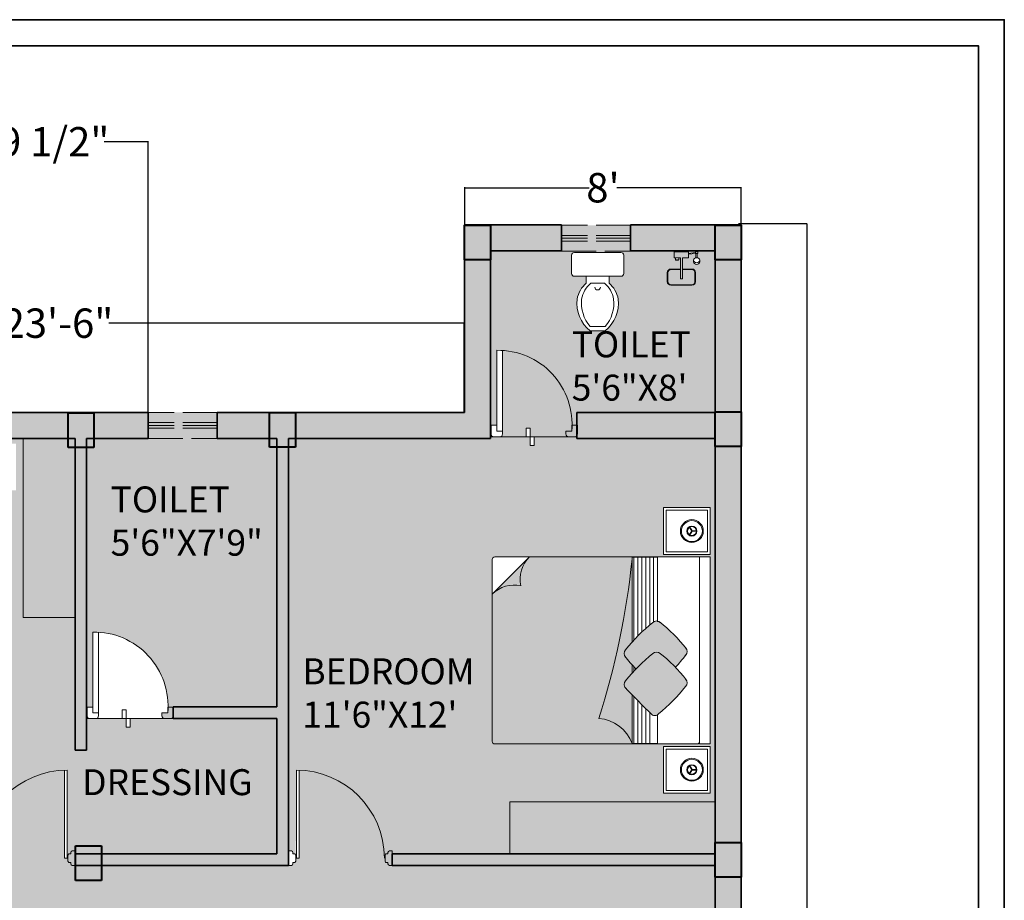
# Model space of a CAD drawing. Units: inches. Extents: x 1077 to 2505, y 1892 to 2728.
# Tile 26 of 26: x 2164 to 2505, y 2423 to 2728. Entities that reach past the tile are written whole.
import ezdxf

# ---------------------------------------------------------------- set-up
doc = ezdxf.new("R2010")
doc.units = ezdxf.units.IN
doc.linetypes.add('ACAD_ISO02W100', pattern=[15, 12, -3])
doc.layers.get('Defpoints').update_dxf_attribs({"color": 220, "linetype": 'ACAD_ISO02W100'})
for name, color, linetype, lineweight in [('00 FURNITURE', 15, 'Continuous', 15), ('A-ANNO-DIMS', 2, 'Continuous', 18), ('A-ANNO-TTLB', 7, 'Continuous', 35), ('A-AREA-IDEN', 7, 'Continuous', 18), ('A-COLS', 7, 'Continuous', 40), ('A-DOOR', 4, 'Continuous', 18), ('A-FLOR-CASE', 8, 'Continuous', 18), ('A-FLOR-FIXT', 8, 'Continuous', 13), ('A-GLAZ-VENT', 6, 'ACAD_ISO02W100', 13), ('A-WALL-PATT', 7, 'Continuous', 9), ('A_FUR 1', 5, 'Continuous', 5), ('WALL', 7, 'Continuous', 35)]:
    doc.layers.add(name, color=color, linetype=linetype, lineweight=lineweight)
for name, color, linetype, lineweight, true_color in [('A-FLOR-CASE-PATT', 32, 'Continuous', 9, 0xcd6928), ('A-FLOR-PATT', 254, 'Continuous', 9, 0xd7ebd2), ('A-FURN-PATT', 177, 'Continuous', 9, 0x293189)]:
    doc.layers.add(name, color=color, linetype=linetype, lineweight=lineweight, true_color=true_color)
doc.styles.get("Standard").update_dxf_attribs({"font": 'arial.ttf'})
doc.dimstyles.get("Standard").update_dxf_attribs({"dimtxt": 10.18, "dimasz": 0.18, "dimexe": 0.18, "dimexo": 0.0625, "dimgap": 0.09, "dimtad": 0, "dimtih": 1, "dimtoh": 1, "dimdec": 0, "dimzin": 0, "dimdsep": 46, "dimlunit": 3, "dimtxsty": 'Standard', "dimcen": 0.09, "dimadec": 0, "dimazin": 0, "dimtfac": 1, "dimtdec": 0, "dimtofl": 0, "dimtmove": 0, "dimatfit": 3, "dimfxl": 1, "dimtolj": 1, "dimtzin": 0, "dimarcsym": 0})

# ---------------------------------------------------------------- blocks, each defined once
blk = doc.blocks.new('*D20')
at = {"layer": 'A-ANNO-DIMS', "color": 0, "lineweight": -2, "transparency": 16777216}
for p, q in [((2317.98, 2657.32), (2317.98, 2670.23)), ((2318.16, 2670.05), (2361.12, 2670.05)), ((2413.64, 2670.05), (2370.68, 2670.05)), ((2413.82, 2657.32), (2413.82, 2670.23))]:
    blk.add_line(p, q, dxfattribs=at)
at = {"layer": 'A-ANNO-DIMS', "color": 0, "transparency": 16777216}
for points in [[(2318.16, 2670.08), (2318.16, 2670.02), (2317.98, 2670.05)], [(2413.64, 2670.08), (2413.64, 2670.02), (2413.82, 2670.05)]]:
    blk.add_solid(points, dxfattribs=at)
at = {"layer": 'Defpoints', "color": 0, "transparency": 16777216}
for p in [(2413.82, 2670.05), (2317.98, 2657.26), (2413.82, 2657.26)]:
    blk.add_point(p, dxfattribs=at)
at = {"layer": 'A-ANNO-DIMS', "color": 0, "transparency": 16777216, "insert": (2365.9, 2670.05), "char_height": 10.18, "attachment_point": 5}
blk.add_mtext("\\A1;8'", dxfattribs=at)
blk = doc.blocks.new('DDD')
at = {"layer": '00 FURNITURE'}
for p, q in [((-12579.77, -15859.53), (-12579.77, -15829.05)), ((-12578.77, -15859.53), (-12578.77, -15829.03)), ((-12612.02, -15857.03), (-12612.02, -15862.03)), ((-12611.02, -15857.03), (-12612.02, -15857.03)), ((-12610.52, -15858.03), (-12610.52, -15857.53)), ((-12577.52, -15858.03), (-12577.52, -15857.53)), ((-12577.02, -15857.03), (-12576.02, -15857.03)), ((-12576.02, -15857.03), (-12576.02, -15862.03)), ((-12610.52, -15861.53), (-12610.52, -15861.03)), ((-12578.77, -15859.53), (-12579.77, -15859.53)), ((-12577.52, -15861.53), (-12577.52, -15861.03)), ((-12612.02, -15862.03), (-12611.02, -15862.03)), ((-12576.02, -15862.03), (-12577.02, -15862.03))]:
    blk.add_line(p, q, dxfattribs=at)
for points in [[(-12610.52, -15861.03), (-12610.02, -15861.03, 0.414214), (-12609.52, -15860.53), (-12609.52, -15858.53, 0.414214), (-12610.02, -15858.03), (-12610.52, -15858.03)], [(-12577.52, -15861.03), (-12578.02, -15861.03, -0.414214), (-12578.52, -15860.53), (-12578.52, -15858.53, -0.414214), (-12578.02, -15858.03), (-12577.52, -15858.03)]]:
    blk.add_lwpolyline(points, format="xyb", dxfattribs=at)
for centre, radius, start, end in [((-12578.77, -15859.53), 30.5, 90, 180), ((-12611.02, -15857.53), 0.5, 0, 90), ((-12577.02, -15857.53), 0.5, 90, 180), ((-12611.02, -15861.53), 0.5, 270, 0), ((-12577.02, -15861.53), 0.5, 180, 270)]:
    blk.add_arc(centre, radius, start, end, dxfattribs=at)
blk = doc.blocks.new('ESTSET')
at = {"layer": 'A_FUR 1'}
for p, q in [((-10.44, 4.1), (-10.44, 32.1)), ((-8.44, 4.1), (-8.44, 32.1)), ((-36.44, 6.1), (-36.44, 3.1)), ((-34.44, 6.1), (-36.44, 6.1)), ((-34.44, 4.1), (-34.44, 6.1)), ((-34.44, 4.1), (-34.44, 6.1)), ((-32.44, 4.1), (-34.44, 4.1)), ((-32.44, 4.1), (-34.44, 4.1)), ((-32.44, 3.1), (-32.44, 4.1)), ((-10.44, 3.1), (-10.44, 4.1)), ((-10.44, 4.1), (-8.44, 4.1)), ((-10.44, 4.1), (-8.44, 4.1)), ((-8.44, 4.1), (-8.44, 6.1)), ((-8.44, 6.1), (-6.44, 6.1)), ((-8.44, 4.1), (-8.44, 6.1)), ((-6.44, 6.1), (-6.44, 3.1)), ((-6.44, 2.1), (-36.44, 2.1)), ((-35.44, 2.1), (-33.44, 2.1)), ((-7.44, 2.1), (-9.44, 2.1))]:
    blk.add_line(p, q, dxfattribs=at)
for points in [[(-21.44, 2.1), (-18.67, 2.1), (-18.67, 5.1), (-20.06, 5.1)], [(-20.06, 5.1), (-20.06, -0.91)], [(-21.44, 2.1), (-21.44, -0.91), (-20.06, -0.91)]]:
    blk.add_lwpolyline(points, dxfattribs=at)
for centre, radius, start, end in [((-8.91, 6.46), 25.64, 88.9606, 185.2816), ((-35.44, 3.1), 1, 180, 270), ((-33.44, 3.1), 1, 270, 0), ((-9.44, 3.1), 1, 180, 270), ((-7.44, 3.1), 1, 270, 0)]:
    blk.add_arc(centre, radius, start, end, dxfattribs=at)
blk = doc.blocks.new('A$C2AC94788')
for p, q in [((0, 0.505), (0, 0.665)), ((0.025, 0.69), (0.435, 0.69)), ((0.46, 0.665), (0.46, 0.505)), ((0.435, 0.48), (0.025, 0.48)), ((0.13, 0.48), (0.13, 0.42)), ((0.33, 0.42), (0.33, 0.48)), ((0.17, 0.42), (0.29, 0.42)), ((0.1641, 0.0392), (0.2959, 0.0392)), ((0.2291, 0.0392), (0.23, 0.0392)), ((0.2309, 0.0392), (0.23, 0.0392)), ((0.165, 0), (0.295, 0))]:
    blk.add_line(p, q)
for centre, radius, start, end in [((0.025, 0.665), 0.025, 90, 180), ((0.435, 0.665), 0.025, 0, 90), ((0.025, 0.505), 0.025, 180, 270), ((0.435, 0.505), 0.025, 270, 0), ((0.2874, 0.2356), 0.2425, 130.48854, 169.44501), ((0.3274, 0.2356), 0.2425, 130.48854, 169.44501), ((0.23, 0.385), 0.025, 180, 0), ((0.1326, 0.2356), 0.2425, 10.55499, 49.51146), ((0.1726, 0.2356), 0.2425, 10.55499, 49.51146), ((0.3601, 0.2448), 0.313, 173.53688, 231.44828), ((0.4001, 0.2448), 0.313, 173.53688, 221.06038), ((0.0999, 0.2448), 0.313, 308.55172, 6.46312), ((0.0599, 0.2448), 0.313, 318.93962, 6.46312)]:
    blk.add_arc(centre, radius, start, end)
blk = doc.blocks.new('A$C7A0926BE')
for p, q in [((-6.55, 0), (-5.57, 0)), ((-6.55, -0.65), (-6.55, 0)), ((-5.57, 0), (-5.57, -0.65)), ((-2.89, 0), (-2.89, -2.29)), ((2.89, 0), (-2.89, 0)), ((2.89, -2.29), (2.89, 0)), ((-7.32, -3.29), (-7.32, -3.94)), ((-5.57, -0.65), (-6.55, -0.65)), ((-6.34, -0.65), (-5.74, -0.65)), ((-6.34, -2.33), (-6.34, -0.65)), ((-5.74, -2.33), (-6.34, -2.33)), ((-5.74, -0.65), (-5.74, -2.33)), ((-5.57, -0.28), (-2.89, -0.56)), ((-5.57, -0.65), (-2.89, -0.94)), ((-4.84, -3.94), (-4.85, -3.29)), ((-2.89, -2.29), (-0.45, -2.29)), ((0.39, -2.29), (2.89, -2.29)), ((1.04, -2.29), (1.04, -3.12)), ((2.37, -2.29), (1.04, -2.29)), ((1.04, -3.12), (2.37, -3.12)), ((1.13, -3.12), (1.13, -3.23)), ((2.3, -3.12), (1.13, -3.12)), ((1.13, -3.23), (2.3, -3.23)), ((2.3, -3.23), (2.3, -3.12)), ((2.37, -3.12), (2.37, -2.29))]:
    blk.add_line(p, q)
at = {"ltscale": 100}
for p, q in [((-0.45, -10.48), (-0.45, -2.29)), ((0.39, -10.48), (0.39, -2.29)), ((0.18, -10.69), (-0.24, -10.69))]:
    blk.add_line(p, q, dxfattribs=at)
for points in [[(-0.45, -6.79), (-4.23, -6.79, 0.414214), (-5.63, -8.19), (-5.63, -11.8, 0.414214), (-4.23, -13.2), (4.17, -13.2, 0.414214), (5.57, -11.8), (5.57, -8.19, 0.414214), (4.17, -6.79), (0.39, -6.79)], [(-0.45, -7), (-4.23, -7, 0.414214), (-5.42, -8.19), (-5.42, -11.8, 0.414214), (-4.23, -12.99), (4.17, -12.99, 0.414214), (5.36, -11.8), (5.36, -8.19, 0.414214), (4.17, -7), (0.39, -7)]]:
    blk.add_lwpolyline(points, format="xyb", dxfattribs=at)
for centre, start, end in [((-0.24, -10.48), 180, 270), ((0.18, -10.48), 270, 0)]:
    blk.add_arc(centre, 0.21, start, end, dxfattribs=at)
at = {"extrusion": (0, 0, -1)}
blk.add_ellipse((-6.08, -3.29), major_axis=(-1.24, 0), ratio=0.790849, dxfattribs=at)
blk.add_ellipse((-6.08, -3.94), major_axis=(-1.24, 0), ratio=0.790849, start_param=3.141593, end_param=6.283185, dxfattribs=at)
blk = doc.blocks.new('RGWTG')
at = {"layer": '00 FURNITURE'}
for p, q in [((578.23, 3473.51), (577.36, 3475.01)), ((578.23, 3473.58), (577.36, 3472.08)), ((578.36, 3473.58), (577.49, 3475.09)), ((578.36, 3473.51), (577.49, 3472)), ((578.29, 3473.62), (580.03, 3473.62)), ((578.29, 3473.47), (580.03, 3473.47)), ((521.93, 3464.58), (509.03, 3451.68)), ((509.03, 3422.63), (509.03, 3463.68)), ((509.93, 3464.58), (566.4, 3464.58)), ((557.53, 3463.84), (557.53, 3464.49)), ((557.53, 3464.49), (566.4, 3464.49)), ((558.2, 3464.49), (558.2, 3435.82)), ((559.57, 3464.49), (559.57, 3437.25)), ((560.94, 3464.49), (560.94, 3438.58)), ((562.3, 3464.49), (562.3, 3439.83)), ((563.67, 3464.49), (563.67, 3440.99)), ((565.04, 3464.49), (565.04, 3442.08)), ((566.4, 3464.58), (580.98, 3464.58)), ((566.4, 3464.49), (566.4, 3442.08)), ((566.4, 3464.49), (566.4, 3463.84)), ((580.98, 3464.58), (580.98, 3416.72)), ((558.2, 3426.48), (558.2, 3425.04)), ((509.03, 3400.68), (509.03, 3422.63)), ((558.2, 3416.13), (558.2, 3399.95)), ((559.57, 3414.75), (559.57, 3399.95)), ((580.98, 3416.72), (580.98, 3400.68)), ((560.94, 3413.39), (560.94, 3399.95)), ((562.3, 3412.04), (562.3, 3399.95)), ((563.67, 3410.72), (563.67, 3399.95)), ((580.08, 3399.78), (509.93, 3399.78)), ((557.53, 3399.95), (557.53, 3400.6)), ((566.4, 3399.95), (557.53, 3399.95)), ((566.4, 3400.6), (566.4, 3399.95)), ((578.23, 3390.78), (577.36, 3392.29)), ((578.23, 3390.86), (577.36, 3389.36)), ((578.36, 3390.86), (577.49, 3392.36)), ((578.29, 3390.9), (580.03, 3390.9)), ((578.36, 3390.78), (577.49, 3389.28)), ((578.29, 3390.74), (580.03, 3390.74))]:
    blk.add_line(p, q, dxfattribs=at)
for points in [[(568.43, 3465.48), (584.63, 3465.48), (584.63, 3481.68), (568.43, 3481.68)], [(569.33, 3466.38), (583.73, 3466.38), (583.73, 3480.78), (569.33, 3480.78)], [(580.98, 3399.78), (584.63, 3399.78), (584.63, 3464.58), (580.98, 3464.58)], [(568.43, 3398.88), (584.63, 3398.88), (584.63, 3382.68), (568.43, 3382.68)], [(569.33, 3397.98), (583.73, 3397.98), (583.73, 3383.58), (569.33, 3383.58)]]:
    blk.add_lwpolyline(points, close=True, dxfattribs=at)
for points in [[(566.52, 3464.49), (557.53, 3464.49), (557.53, 3435.08)], [(557.53, 3427.21), (557.53, 3424.3)], [(557.53, 3416.82), (557.53, 3399.95), (566.4, 3399.95), (566.4, 3409.94)]]:
    blk.add_lwpolyline(points, dxfattribs=at)
for centre, radius in [((578.29, 3473.54), 3.97), ((578.29, 3473.54), 3.63), ((578.29, 3473.54), 1.74), ((578.29, 3473.54), 1.56), ((578.29, 3390.82), 3.97), ((578.29, 3390.82), 3.63), ((578.29, 3390.82), 1.74), ((578.29, 3390.82), 1.56)]:
    blk.add_circle(centre, radius, dxfattribs=at)
for centre, radius, start, end in [((509.93, 3463.68), 0.9, 90, 180), ((529.65, 3456.88), 10.9, 135.0361, 191.9278), ((290.56, 3490.52), 268.3, 342.2214, 354.2925), ((516.73, 3443.97), 10.9, 78.0722, 134.9639), ((566.05, 3440.57), 1.82, 45, 135), ((533.58, 3399.31), 54.32, 37.931, 52.069), ((598.15, 3399.01), 54.32, 127.931, 142.069), ((556.59, 3431.11), 1.82, 135, 225), ((574.84, 3431.77), 1.82, 315, 45), ((597.87, 3463.6), 54.32, 217.931, 224.141), ((598.15, 3388.23), 54.32, 127.931, 142.069), ((566.05, 3429.78), 1.82, 45, 135), ((533.58, 3388.53), 54.32, 37.931, 52.069), ((533.28, 3463.88), 54.32, 316.32, 322.069), ((556.59, 3420.33), 1.82, 135, 225), ((574.84, 3420.99), 1.82, 315, 45), ((765.33, 3619.75), 290.45, 223.6069, 226.2326), ((533.28, 3453.1), 54.32, 307.931, 322.069), ((545.02, 3395.29), 13.35, 20.4224, 85.5825), ((565.44, 3411.05), 1.47, 225.9674, 326.8337), ((509.93, 3400.68), 0.9, 180, 270), ((580.08, 3400.68), 0.9, 270, 0)]:
    blk.add_arc(centre, radius, start, end, dxfattribs=at)
blk = doc.blocks.new('C1')
h = blk.add_hatch(color=256)
h.dxf.hatch_style = 1
h.paths.add_polyline_path([(1668.56, 2445.41), (1677.56, 2445.41), (1677.56, 2457.41), (1668.56, 2457.41)])
for p, q in [((1668.56, 2457.41), (1677.56, 2457.41)), ((1668.56, 2445.41), (1668.56, 2457.41)), ((1677.56, 2457.41), (1677.56, 2445.41)), ((1677.56, 2445.41), (1668.56, 2445.41))]:
    blk.add_line(p, q)
blk = doc.blocks.new('*D18')
at = {"layer": 'A-ANNO-DIMS', "color": 0, "lineweight": -2, "transparency": 16777216}
for p, q in [((2035.96, 2592.42), (2035.96, 2623.29)), ((2036.14, 2623.11), (2159.23, 2623.11)), ((2317.64, 2623.11), (2194.55, 2623.11)), ((2317.82, 2592.42), (2317.82, 2623.29))]:
    blk.add_line(p, q, dxfattribs=at)
at = {"layer": 'A-ANNO-DIMS', "color": 0, "transparency": 16777216}
for points in [[(2036.14, 2623.14), (2036.14, 2623.08), (2035.96, 2623.11)], [(2317.64, 2623.14), (2317.64, 2623.08), (2317.82, 2623.11)]]:
    blk.add_solid(points, dxfattribs=at)
at = {"layer": 'Defpoints', "color": 0, "transparency": 16777216}
for p in [(2317.82, 2623.11), (2035.96, 2592.36), (2317.82, 2592.36)]:
    blk.add_point(p, dxfattribs=at)
at = {"layer": 'A-ANNO-DIMS', "color": 0, "transparency": 16777216, "insert": (2176.89, 2623.11), "char_height": 10.18, "attachment_point": 5}
blk.add_mtext('\\A1;23\'-6"', dxfattribs=at)
blk = doc.blocks.new('*D19')
at = {"layer": 'A-ANNO-DIMS', "color": 0, "lineweight": -2, "transparency": 16777216}
for p, q in [((2412.91, 2657.64), (2436.75, 2657.64)), ((2436.57, 2657.46), (2436.57, 2381.28)), ((2436.57, 2094.52), (2436.57, 2370.7)), ((2412.91, 2094.34), (2436.75, 2094.34))]:
    blk.add_line(p, q, dxfattribs=at)
at = {"layer": 'A-ANNO-DIMS', "color": 0, "transparency": 16777216}
for points in [[(2436.54, 2657.46), (2436.6, 2657.46), (2436.57, 2657.64)], [(2436.54, 2094.52), (2436.6, 2094.52), (2436.57, 2094.34)]]:
    blk.add_solid(points, dxfattribs=at)
at = {"layer": 'Defpoints', "color": 0, "transparency": 16777216}
for p in [(2412.85, 2657.64), (2412.85, 2094.34), (2436.57, 2094.34)]:
    blk.add_point(p, dxfattribs=at)
at = {"layer": 'A-ANNO-DIMS', "color": 0, "transparency": 16777216, "insert": (2436.57, 2375.99), "char_height": 10.18, "attachment_point": 5}
blk.add_mtext('\\A1;46\'-11"', dxfattribs=at)
blk = doc.blocks.new('VENT-24')
for p, q in [((3.5, 24), (3.5, 0)), ((4.5, 24), (4.5, 0)), ((5.5, 24), (5.5, 0))]:
    blk.add_line(p, q)
blk.add_lwpolyline([(0, 0), (9, 0), (9, 24), (0, 24)], close=True)
blk = doc.blocks.new('SHEET-FRAME-RESIDENTIAL')
for points in [[(0, 830.04), (543.52, 830.04), (543.52, 0), (0, 0)], [(9, 821.04), (534.52, 821.04), (534.52, 9), (9, 9)]]:
    blk.add_lwpolyline(points, close=True)
blk = doc.blocks.new('*D48')
at = {"layer": 'A-ANNO-DIMS', "color": 0, "lineweight": -2, "transparency": 16777216}
for p, q in [((2256.78, 2416.24), (2259.43, 2416.24)), ((2259.25, 2416.06), (2259.25, 2413.13)), ((2259.25, 2399.49), (2259.25, 2402.42)), ((2256.78, 2399.31), (2259.43, 2399.31))]:
    blk.add_line(p, q, dxfattribs=at)
at = {"layer": 'A-ANNO-DIMS', "color": 0, "transparency": 16777216}
for points in [[(2259.22, 2416.06), (2259.28, 2416.06), (2259.25, 2416.24)], [(2259.22, 2399.49), (2259.28, 2399.49), (2259.25, 2399.31)]]:
    blk.add_solid(points, dxfattribs=at)
at = {"layer": 'Defpoints', "color": 0, "transparency": 16777216}
for p in [(2256.72, 2416.24), (2259.25, 2416.24), (2256.72, 2399.31)]:
    blk.add_point(p, dxfattribs=at)
at = {"layer": 'A-ANNO-DIMS', "color": 0, "transparency": 16777216, "insert": (2259.25, 2407.77), "char_height": 10.18, "attachment_point": 5}
blk.add_mtext('\\A1;DINING CHAIR 1\'-5" TYP.', dxfattribs=at)
blk = doc.blocks.new('*D74')
at = {"layer": 'A-ANNO-DIMS', "color": 0, "lineweight": -2, "transparency": 16777216}
for p, q in [((2126.63, 2592.2), (2126.63, 2686.17)), ((2126.81, 2685.99), (2141.88, 2685.99)), ((2207.97, 2685.99), (2192.9, 2685.99)), ((2208.15, 2592.2), (2208.15, 2686.17))]:
    blk.add_line(p, q, dxfattribs=at)
at = {"layer": 'A-ANNO-DIMS', "color": 0, "transparency": 16777216}
for points in [[(2126.81, 2686.02), (2126.81, 2685.96), (2126.63, 2685.99)], [(2207.97, 2686.02), (2207.97, 2685.96), (2208.15, 2685.99)]]:
    blk.add_solid(points, dxfattribs=at)
at = {"layer": 'Defpoints', "color": 0, "transparency": 16777216}
for p in [(2208.15, 2685.99), (2126.63, 2592.14), (2208.15, 2592.14)]:
    blk.add_point(p, dxfattribs=at)
at = {"layer": 'A-ANNO-DIMS', "color": 0, "transparency": 16777216, "insert": (2167.39, 2685.99), "char_height": 10.18, "attachment_point": 5}
blk.add_mtext('\\A1;6\'-9 1/2"', dxfattribs=at)

msp = doc.modelspace()

# ---------------------------------------------------------------- hatches: boundary and pattern name
at = {"layer": 'A-FLOR-CASE-PATT', "transparency": 33554610}
h = msp.add_hatch(color=256, dxfattribs=at)
h.dxf.hatch_style = 1
h.paths.add_polyline_path([(2182.85, 2583.13), (2164.84, 2583.13), (2164.84, 2521.11), (2182.85, 2521.11)])
h.paths.add_polyline_path([(2333.66, 2457.16), (2333.66, 2439.14), (2404.85, 2439.14), (2404.85, 2443.09), (2404.85, 2457.16)])
at = {"layer": 'A-FLOR-PATT', "transparency": 33554559}
h = msp.add_hatch(color=256, dxfattribs=at)
h.dxf.hatch_style = 1
h.paths.add_polyline_path([(2252.85, 2583.14), (2232.15, 2583.14), (2208.15, 2583.17), (2208.15, 2583.14), (2186.85, 2583.14), (2186.85, 2486.14), (2186.85, 2475.14), (2182.85, 2475.14), (2182.85, 2521.11), (2164.84, 2521.11), (2164.84, 2583.14), (2126.63, 2583.14), (2078.63, 2583.13), (2078.63, 2583.14), (2044.85, 2583.14), (2044.85, 2439.14), (2146.85, 2439.14), (2146.85, 2435.14), (2120.85, 2435.14), (2044.85, 2435.14), (2044.85, 2401), (2044.85, 2401), (2044.85, 2377), (2044.85, 2377), (2044.85, 2313.14), (2116.85, 2313.14), (2116.85, 2405.14), (2120.85, 2405.14), (2120.85, 2313.14), (2146.85, 2313.14), (2146.85, 2312.21), (2182.85, 2312.21), (2182.85, 2313.14), (2186.85, 2313.14), (2186.85, 2312.21), (2222.85, 2312.21), (2222.85, 2313.14), (2289.85, 2313.14), (2289.85, 2094.14), (2404.85, 2094.14), (2404.85, 2146.06), (2368.85, 2146.06), (2368.85, 2273.14), (2332.85, 2273.14), (2332.85, 2309.14), (2325.85, 2309.14), (2325.85, 2313.14), (2404.85, 2313.14), (2404.85, 2354.2), (2404.85, 2402.2), (2404.85, 2435.14), (2292.85, 2435.14), (2292.85, 2439.14), (2333.66, 2439.14), (2333.66, 2457.16), (2404.85, 2457.16), (2404.85, 2583.14), (2356.85, 2583.14), (2356.85, 2592.14), (2404.85, 2592.14), (2404.85, 2648.14), (2375.5, 2648.14), (2375.5, 2648.03), (2351.47, 2648.03), (2351.47, 2648.14), (2326.85, 2648.14), (2326.85, 2583.14), (2256.85, 2583.14), (2256.85, 2435.14), (2182.85, 2435.14), (2182.85, 2439.14), (2186.85, 2439.14), (2252.85, 2439.14), (2252.85, 2486.14), (2216.85, 2486.14), (2216.85, 2490.14), (2252.85, 2490.14)])
h.paths.add_polyline_path([(2214.97, 2488.05), (2212.97, 2488.05), (2212.97, 2487.05, 0.414214), (2213.97, 2486.05), (2201.97, 2486.05), (2201.97, 2483.04), (2200.58, 2483.04), (2200.58, 2486.05), (2187.97, 2486.05, -0.414214), (2186.97, 2487.05), (2186.97, 2490.05), (2188.97, 2490.05), (2188.97, 2516.05, -0.446908)], flags=16)
h.paths.add_polyline_path([(2162.4, 2565.16), (2146.2, 2565.16), (2146.2, 2581.36), (2162.4, 2581.36)], flags=16)
h.paths.add_polyline_path([(2161.5, 2566.06), (2147.1, 2566.06), (2147.1, 2580.46), (2161.5, 2580.46)], flags=0)
h.paths.add_polyline_path([(2145.3, 2506.66, -0.414214), (2144.4, 2505.76), (2122.45, 2505.76), (2081.4, 2505.76, -0.414214), (2080.5, 2506.66), (2080.5, 2563.14), (2080.5, 2577.72), (2080.5, 2581.36), (2145.3, 2581.36), (2145.3, 2577.72), (2144.4, 2577.72, -0.414214), (2145.3, 2576.82)], flags=16)
h.paths.add_polyline_path([(2150.3, 2575.03, -1), (2158.24, 2575.03, -1)], flags=0)
h.paths.add_polyline_path([(2150.64, 2575.03, -1), (2157.89, 2575.03, -1)], flags=0)
h.paths.add_polyline_path([(2180.11, 2468.19), (2180.11, 2437.69), (2180.36, 2436.69), (2180.36, 2437.69), (2179.11, 2437.69), (2179.11, 2468.17, 0.404641), (2149.61, 2437.69), (2149.36, 2436.69, -0.414214), (2148.86, 2436.19), (2148.36, 2436.19), (2148.36, 2435.69, -0.414214), (2147.86, 2435.19), (2146.86, 2435.19), (2146.86, 2440.19), (2147.86, 2440.19, -0.414214), (2148.36, 2439.69), (2148.36, 2439.19), (2148.86, 2439.19, -0.414214), (2149.36, 2438.69), (2149.61, 2437.69, -0.414214)], flags=16)
h.paths.add_polyline_path([(2145.14, 2554.26, 0.292232), (2136.49, 2542.78, 0.052719), (2081.25, 2554.26), (2080.6, 2554.26), (2080.6, 2563.14), (2081.25, 2563.14), (2102.73, 2563.14, -0.117785), (2103.09, 2563.91, -0.059418), (2112.19, 2573, -0.379859), (2114.6, 2572.86, -0.02509), (2118.73, 2569.3, -0.025935), (2122.97, 2573, -0.379859), (2125.38, 2572.86, -0.061767), (2134.84, 2563.41, -0.069393), (2135.14, 2563.14), (2145.14, 2563.14)], flags=0)
h.paths.add_polyline_path([(2120.79, 2554.26), (2117.88, 2554.26, -0.015371), (2115.33, 2552.11, -0.429576), (2112.69, 2552.04, -0.016036), (2110.01, 2554.26), (2080.6, 2554.26), (2080.6, 2560.4), (2104.1, 2560.4, 0.055344), (2112.69, 2552.04, 0.331768), (2114.84, 2551.72, 0.027343), (2119.32, 2555.62, 0.00919)], flags=0)
h.paths.add_polyline_path([(2152.88, 2574.32), (2154.19, 2575.07), (2154.19, 2576.58, 0.399698), (2152.71, 2575.03, 0.119004)], flags=0)
h.paths.add_polyline_path([(2152.53, 2575.03, -1), (2156, 2575.03, -1)], flags=0)
h.paths.add_polyline_path([(2154.27, 2574.94), (2154.34, 2574.98), (2154.34, 2575.07), (2154.3, 2575.09), (2154.23, 2574.96)], flags=0)
h.paths.add_polyline_path([(2259.6, 2468.17, -0.414214), (2290.1, 2437.67), (2290.35, 2438.67), (2290.1, 2437.67, 0.404641), (2260.6, 2468.15), (2260.6, 2437.67), (2259.35, 2437.67), (2259.35, 2436.67, -0.414214), (2258.85, 2436.17), (2258.35, 2436.17), (2258.35, 2435.67, -0.414214), (2257.85, 2435.17), (2256.85, 2435.17), (2256.85, 2440.17), (2257.85, 2440.17, -0.414214), (2258.35, 2439.67), (2258.35, 2439.17), (2258.85, 2439.17, -0.414214), (2259.35, 2438.67)], flags=16)
h.paths.add_polyline_path([(2327.48, 2541.19, -0.414214), (2328.38, 2542.09), (2384.85, 2542.09), (2399.43, 2542.09), (2403.08, 2542.09), (2403.08, 2477.29), (2399.43, 2477.29), (2399.43, 2478.19, -0.414214), (2398.53, 2477.29), (2328.38, 2477.29, -0.414214), (2327.48, 2478.19), (2327.48, 2500.14)], flags=16)
h.paths.add_polyline_path([(2340.38, 2542.09, 0.253465), (2337.43, 2532.13, 0.2538), (2327.47, 2529.17)], flags=16)
h.paths.add_polyline_path([(2080.5, 2518.67, 0.253465), (2090.46, 2515.72, 0.2538), (2093.42, 2505.75)], flags=16)
h.paths.add_polyline_path([(2327.09, 2584.7), (2327.09, 2587.7), (2329.09, 2587.7), (2329.09, 2613.7, -0.01951), (2331.09, 2613.66), (2331.09, 2585.7), (2331.09, 2584.7, -0.414214), (2330.09, 2583.7), (2328.09, 2583.7, -0.414214)], flags=16)
h.paths.add_polyline_path([(2239.78, 2404.11), (2252.36, 2404.11), (2252.36, 2405.72), (2239.78, 2405.72)], flags=16)
h.paths.add_polyline_path([(2237.26, 2403.16), (2237.26, 2395.8), (2237.82, 2395.8), (2237.82, 2402.03, -0.41429), (2238.38, 2402.59), (2253.79, 2402.59, -0.414213), (2254.35, 2402.03), (2254.35, 2395.8), (2254.91, 2395.8), (2254.91, 2403.16)], flags=16)
h.paths.add_polyline_path([(2120.69, 2434.12), (2120.69, 2432.12, -0.414214), (2119.69, 2431.12), (2118.69, 2431.12), (2090.73, 2431.12, 0.400854), (2116.69, 2407.02), (2116.69, 2407.12), (2118.69, 2407.12, -0.446908), (2090.69, 2433.12), (2116.69, 2433.12), (2116.69, 2435.12), (2119.69, 2435.12, -0.414214)], flags=16)
h.paths.add_polyline_path([(2262.11, 2404.11), (2274.69, 2404.11), (2274.69, 2405.72), (2262.11, 2405.72)], flags=16)
h.paths.add_polyline_path([(2259.59, 2403.16), (2262.11, 2404.11), (2274.69, 2404.11), (2277.24, 2403.16)], flags=16)
h.paths.add_polyline_path([(2289.58, 2389.14), (2289.58, 2376.57), (2291.19, 2376.57), (2291.19, 2389.14)], flags=16)
h.paths.add_polyline_path([(2288.62, 2391.67), (2281.15, 2391.67), (2281.15, 2391.11), (2287.5, 2391.11, -0.41429), (2288.06, 2390.54), (2288.06, 2375.14, -0.414237), (2287.5, 2374.58), (2281.15, 2374.58), (2281.15, 2374.01), (2288.62, 2374.01)], flags=16)
h.paths.add_polyline_path([(2274.69, 2357.14), (2274.69, 2355.52), (2276.22, 2355.52, 0.414236), (2277.24, 2356.54), (2277.24, 2358.09)], flags=16)
h.paths.add_polyline_path([(2252.36, 2357.14), (2252.36, 2355.52), (2253.89, 2355.52, 0.414235), (2254.91, 2356.54), (2254.91, 2358.09)], flags=16)
h.paths.add_polyline_path([(2224.02, 2376.03), (2222.41, 2376.03), (2222.41, 2374.5, 0.414235), (2223.43, 2373.48), (2224.98, 2373.48)], flags=16)
h.paths.add_polyline_path([(2276.68, 2365.45), (2276.68, 2359.22, -0.41419), (2276.12, 2358.66), (2260.71, 2358.66, -0.414137), (2260.15, 2359.22), (2260.15, 2365.45), (2254.35, 2365.45), (2254.35, 2359.22, -0.414189), (2253.79, 2358.66), (2238.38, 2358.66, -0.414137), (2237.82, 2359.22), (2237.82, 2365.45)], flags=16)
h.paths.add_polyline_path([(2079.6, 2565.16), (2063.4, 2565.16), (2063.4, 2581.36), (2079.6, 2581.36)], flags=16)
h.paths.add_polyline_path([(2078.7, 2566.06), (2064.3, 2566.06), (2064.3, 2580.46), (2078.7, 2580.46)], flags=0)
h.paths.add_polyline_path([(2339.31, 2583.7), (2339.31, 2586.71), (2340.7, 2586.71), (2340.7, 2583.7), (2342.09, 2583.7), (2342.09, 2580.7), (2340.7, 2580.7), (2340.7, 2583.7)], flags=16)
h.paths.add_polyline_path([(2123.69, 2421.51), (2123.69, 2420.12), (2120.69, 2420.12), (2120.69, 2421.51), (2117.68, 2421.51), (2117.68, 2422.89), (2120.69, 2422.89), (2120.69, 2421.51)], flags=16)
h.paths.add_polyline_path([(2067.57, 2575.03, -1), (2075.51, 2575.03, -1)], flags=0)
h.paths.add_polyline_path([(2067.92, 2575.03, -1), (2075.17, 2575.03, -1)], flags=0)
h.paths.add_polyline_path([(2070.16, 2574.32), (2071.47, 2575.07), (2071.47, 2576.58, 0.399698), (2069.99, 2575.03, 0.119004)], flags=0)
h.paths.add_polyline_path([(2069.81, 2575.03, -1), (2073.28, 2575.03, -1)], flags=0)
h.paths.add_polyline_path([(2071.54, 2574.94), (2071.62, 2574.89), (2071.62, 2574.98)], flags=0)
h.paths.add_polyline_path([(2364.5, 2486.1, 0.052719), (2375.98, 2541.34), (2375.98, 2541.99), (2384.85, 2541.99), (2384.85, 2541.34), (2384.85, 2519.86, -0.117785), (2385.62, 2519.51, -0.059418), (2394.72, 2510.41, -0.379859), (2394.58, 2507.99, -0.02509), (2391.01, 2503.87, -0.025935), (2394.72, 2499.62, -0.379859), (2394.58, 2497.21, -0.061767), (2385.12, 2487.75, -0.069393), (2384.85, 2487.45), (2384.85, 2477.45), (2375.98, 2477.45, 0.292232)], flags=0)
h.paths.add_polyline_path([(2373.75, 2509.9, -0.016036), (2375.98, 2512.58), (2375.98, 2541.99), (2382.12, 2541.99), (2382.12, 2518.49, 0.055344), (2373.75, 2509.9, 0.331768), (2373.44, 2507.75, 0.027343), (2377.33, 2503.27, 0.00919), (2375.98, 2501.8), (2375.98, 2504.71, -0.015371), (2373.82, 2507.26, -0.429576)], flags=0)
h.paths.add_polyline_path([(2356.95, 2631.48, -0.171636), (2360.13, 2636.99), (2360.13, 2639.35), (2356, 2639.35, -0.414214), (2355.01, 2640.34), (2355.01, 2646.64, -0.414214), (2356, 2647.62), (2372.14, 2647.62, -0.414214), (2373.13, 2646.64), (2373.13, 2640.34, -0.414214), (2372.14, 2639.35), (2368.01, 2639.35), (2368.01, 2636.99, -0.171636), (2371.2, 2631.48, -0.258205), (2366.63, 2620.45), (2361.51, 2620.45, -0.258205)], flags=16)
h.paths.add_polyline_path([(2358.52, 2631.48, -0.171636), (2361.71, 2636.99), (2366.43, 2636.99, -0.171636), (2369.62, 2631.48, -0.210384), (2366.67, 2622), (2361.47, 2622, -0.210384)], flags=0)
h.paths.add_polyline_path([(2386.88, 2542.99), (2386.88, 2559.19), (2403.08, 2559.19), (2403.08, 2542.99)], flags=16)
h.paths.add_polyline_path([(2387.78, 2543.89), (2387.78, 2558.29), (2402.18, 2558.29), (2402.18, 2543.89)], flags=0)
h.paths.add_polyline_path([(2392.77, 2551.05, -1), (2400.71, 2551.05, -1)], flags=0)
h.paths.add_polyline_path([(2393.11, 2551.05, -1), (2400.37, 2551.05, -1)], flags=0)
h.paths.add_polyline_path([(2386.88, 2476.39), (2403.08, 2476.39), (2403.08, 2460.19), (2386.88, 2460.19)], flags=16)
h.paths.add_polyline_path([(2398.48, 2550.97), (2398.3, 2550.97, -0.544606), (2396.03, 2549.66), (2395.94, 2549.51, 0.547962)], flags=0)
h.paths.add_polyline_path([(2387.78, 2475.49), (2402.18, 2475.49), (2402.18, 2461.09), (2387.78, 2461.09)], flags=0)
h.paths.add_polyline_path([(2396.79, 2551.12), (2396.74, 2551.2), (2396.7, 2551.12)], flags=0)
h.paths.add_polyline_path([(2400.71, 2468.32, -1), (2392.77, 2468.32, -1)], flags=0)
h.paths.add_polyline_path([(2400.37, 2468.32, -1), (2393.11, 2468.32, -1)], flags=0)
h.paths.add_polyline_path([(2398.48, 2468.25), (2398.3, 2468.25, -0.544606), (2396.03, 2466.94), (2395.94, 2466.78, 0.547962)], flags=0)
h.paths.add_polyline_path([(2396.79, 2468.4), (2396.74, 2468.48), (2396.7, 2468.4)], flags=0)
h.paths.add_polyline_path([(2292.64, 2341.23, -0.414214), (2323.14, 2310.73), (2323.39, 2311.73), (2323.14, 2310.73, 0.404641), (2293.64, 2341.21), (2293.64, 2310.73), (2292.39, 2310.73), (2292.39, 2309.73, -0.414214), (2291.89, 2309.23), (2291.39, 2309.23), (2291.39, 2308.73, -0.414214), (2290.89, 2308.23), (2289.89, 2308.23), (2289.89, 2313.23), (2290.89, 2313.23, -0.414214), (2291.39, 2312.73), (2291.39, 2312.23), (2291.89, 2312.23, -0.414214), (2292.39, 2311.73)], flags=16)
h.paths.add_polyline_path([(2389.45, 2641.69), (2392.75, 2641.69), (2392.75, 2641.87), (2389.45, 2641.87)], flags=16)
edge = h.paths.add_edge_path(flags=16)
edge.add_arc((2393.3, 2638.65), 0.183, 270, 360)
edge.add_line((2393.49, 2638.65), (2393.49, 2645.8))
edge.add_line((2393.49, 2645.8), (2395.61, 2645.8))
edge.add_line((2395.61, 2645.8), (2395.61, 2647.8))
edge.add_line((2395.61, 2647.8), (2390.57, 2647.8))
edge.add_line((2390.57, 2647.8), (2390.57, 2645.8))
edge.add_line((2390.57, 2645.8), (2392.19, 2645.8))
edge.add_line((2392.19, 2645.8), (2392.19, 2644.98))
edge.add_line((2392.19, 2644.98), (2391.02, 2644.98))
edge.add_line((2391.02, 2644.98), (2391.02, 2645.8))
edge.add_line((2391.02, 2645.8), (2390.57, 2645.8))
edge.add_line((2390.57, 2645.8), (2390.57, 2647.8))
edge.add_line((2390.57, 2647.8), (2395.61, 2647.8))
edge.add_line((2395.61, 2647.8), (2395.61, 2647.32))
edge.add_line((2395.61, 2647.32), (2397.95, 2647.56))
edge.add_line((2397.95, 2647.56), (2397.95, 2647.8))
edge.add_line((2397.95, 2647.8), (2398.81, 2647.8))
edge.add_line((2398.81, 2647.8), (2398.81, 2647.23))
edge.add_line((2398.81, 2647.23), (2398.63, 2645.77))
edge.add_ellipse((2398.41, 2644.93), major_axis=(-1.08, 0), ratio=0.790849, start_angle=180, end_angle=255.2976, ccw=False)
edge.add_line((2399.49, 2644.93), (2399.49, 2644.36))
edge.add_ellipse((2398.41, 2644.36), major_axis=(-1.08, 0), ratio=0.790849, start_angle=0, end_angle=180, ccw=False)
edge.add_line((2397.32, 2644.36), (2397.33, 2644.85))
edge.add_ellipse((2398.41, 2644.93), major_axis=(-1.08, 0), ratio=0.790849, start_angle=284.7024, end_angle=364.0401, ccw=False)
edge.add_line((2398.1, 2645.73), (2398.1, 2647.23))
edge.add_line((2398.1, 2647.23), (2397.95, 2647.23))
edge.add_line((2397.95, 2647.23), (2395.61, 2646.99))
edge.add_line((2395.61, 2646.99), (2395.61, 2645.8))
edge.add_line((2395.61, 2645.8), (2393.49, 2645.8))
edge.add_line((2393.49, 2645.8), (2393.49, 2638.46))
edge.add_line((2393.49, 2638.46), (2393.3, 2638.46))
h.paths.add_polyline_path([(2353.64, 2256.32, -0.292371), (2356.22, 2253.81, -0.085148), (2358.52, 2214.83, -0.01331), (2357.59, 2104.48, -0.379287), (2354.54, 2101.26, -0.0502), (2298.86, 2101.26, -0.379287), (2295.81, 2104.48, -0.01331), (2294.88, 2214.83, -0.086132), (2297.28, 2254.24, -0.295116), (2299.9, 2256.76, -0.114238)], flags=16)
h.paths.add_polyline_path([(2352.48, 2211.82, -0.355389), (2354.02, 2208.08), (2350.26, 2195.63, -0.398275), (2346.44, 2193.45, 0.113332), (2306.96, 2193.45, -0.398275), (2303.14, 2195.63), (2299.38, 2208.08, -0.355394), (2300.92, 2211.82, -0.265725)], flags=0)
h.paths.add_polyline_path([(2297.68, 2201.7), (2303.26, 2187.65), (2303.26, 2166.61), (2298.16, 2163.24)], flags=0)
h.paths.add_polyline_path([(2355.78, 2201.7), (2355.31, 2163.24), (2350.2, 2166.61), (2350.2, 2187.65)], flags=0)
h.paths.add_polyline_path([(2303.26, 2164.35), (2303.26, 2143.1), (2298.44, 2128.54), (2298.19, 2161.01)], flags=0)
h.paths.add_polyline_path([(2350.2, 2164.35), (2355.28, 2161.01), (2355.03, 2128.54), (2350.2, 2143.1)], flags=0)
h.paths.add_polyline_path([(2347.2, 2136.38), (2351.71, 2113.65, -0.090102), (2301.76, 2113.63), (2306.27, 2136.37, 0.036636)], flags=0)
h.paths.add_polyline_path([(2304.86, 2165.32), (2354.76, 2165.32), (2354.76, 2183.87), (2304.86, 2183.87)], flags=8)
h.paths.add_polyline_path([(2053.76, 2360.82), (2103.97, 2360.82), (2103.97, 2394.41), (2053.76, 2394.41)], flags=24)
h.paths.add_polyline_path([(2153.41, 2366.23), (2211.12, 2366.23), (2211.12, 2399.82), (2153.41, 2399.82)], flags=24)
h.paths.add_polyline_path([(2258.04, 2477.83), (2327.95, 2477.83), (2327.95, 2511.42), (2258.04, 2511.42)], flags=24)
h.paths.add_polyline_path([(2182.1, 2454.46), (2252.27, 2454.46), (2252.27, 2473), (2182.1, 2473)], flags=24)
h.paths.add_polyline_path([(2192.4, 2537.41), (2246.99, 2537.41), (2246.99, 2571), (2192.4, 2571)], flags=24)
h.paths.add_polyline_path([(2083.07, 2465.98), (2152.99, 2465.98), (2152.99, 2499.56), (2083.07, 2499.56)], flags=24)
at = {"layer": 'A-FURN-PATT', "transparency": 33554610}
h = msp.add_hatch(color=256, dxfattribs=at)
h.dxf.hatch_style = 1
h.paths.add_polyline_path([(2375.98, 2541.34), (2375.98, 2542.09), (2340.38, 2542.09, 0.253465), (2337.43, 2532.13, 0.253465), (2327.48, 2529.18), (2327.48, 2500.14), (2327.48, 2478.19, 0.414214), (2328.38, 2477.29), (2376.04, 2477.29, 0.295777), (2364.5, 2486.1, 0.052719)])
h.paths.add_polyline_path([(2340.38, 2542.09), (2327.47, 2529.17, -0.2538), (2337.43, 2532.13, -0.253465)])
h.paths.add_polyline_path([(2385.62, 2508.72, 0.379859), (2383.21, 2508.58, 0.061767), (2373.75, 2499.12, 0.334836), (2373.45, 2496.95, 0.011497), (2382.88, 2487.49, 0.468078), (2385.12, 2487.75, 0.061767), (2394.58, 2497.21, 0.380465), (2394.72, 2499.63, 0.059418)])
h.paths.add_polyline_path([(2385.62, 2519.5, 0.379859), (2383.21, 2519.36, 0.061767), (2373.75, 2509.9, 0.331768), (2373.44, 2507.75, 0.027343), (2377.33, 2503.27, -0.036481), (2383.21, 2508.58, -0.379859), (2385.62, 2508.72, -0.033431), (2391.01, 2503.86, 0.025099), (2394.58, 2507.99, 0.380465), (2394.72, 2510.41, 0.059418)])
h.paths.add_polyline_path([(2375.98, 2494.32, -0.003141), (2373.45, 2496.95, -0.334836), (2373.75, 2499.12, -0.016036), (2375.98, 2501.8), (2375.98, 2504.71, -0.015371), (2373.82, 2507.26, -0.429576), (2373.75, 2509.9, -0.016036), (2375.98, 2512.58), (2375.98, 2541.34, -0.052719), (2364.5, 2486.1, -0.292232), (2375.98, 2477.45)], flags=17)
at = {"layer": 'A-WALL-PATT', "transparency": 33554585}
h = msp.add_hatch(color=256, dxfattribs=at)
h.dxf.hatch_style = 1
h.paths.add_polyline_path([(2044.85, 2429.98), (2035.85, 2429.98), (2035.85, 2401), (2044.85, 2401)])
h.paths.add_polyline_path([(2044.85, 2377), (2035.85, 2377), (2035.85, 2317.47), (2044.85, 2317.47)])
h.paths.add_polyline_path([(2085.45, 2159.14), (2044.85, 2159.14), (2044.85, 2225.64), (2035.85, 2225.64), (2035.85, 2106.16), (2044.85, 2106.16), (2044.85, 2150.14), (2085.45, 2150.14)])
h.paths.add_polyline_path([(2289.85, 2103.14), (2044.85, 2103.14), (2044.85, 2106.16), (2035.85, 2106.16), (2035.85, 2094.14), (2289.85, 2094.14)])
h.paths.add_polyline_path([(2413.85, 2354.2), (2404.85, 2354.2), (2404.85, 2354.2), (2404.85, 2313.14), (2325.85, 2313.14), (2325.85, 2309.14), (2404.85, 2309.14), (2404.85, 2094.14), (2413.85, 2094.14)])
h.paths.add_polyline_path([(2413.85, 2431.09), (2404.85, 2431.09), (2404.85, 2402.2), (2413.85, 2402.2)])
h.paths.add_polyline_path([(2404.85, 2439.14), (2292.85, 2439.14), (2292.85, 2435.14), (2404.85, 2435.14)])
h.paths.add_polyline_path([(2413.85, 2580.36), (2404.85, 2580.36), (2404.85, 2457.16), (2404.87, 2457.16), (2404.87, 2443.09), (2413.85, 2443.09)])
h.paths.add_polyline_path([(2413.85, 2645.09), (2404.85, 2645.09), (2404.85, 2592.36), (2413.85, 2592.36)])
h.paths.add_polyline_path([(2413.85, 2645.09), (2404.85, 2645.09), (2404.85, 2648.14), (2375.5, 2648.14), (2375.5, 2648.03), (2351.5, 2648.03), (2351.5, 2657.03), (2375.47, 2657.03), (2375.47, 2657.14), (2413.85, 2657.14)])
h.paths.add_polyline_path([(2351.47, 2657.14), (2326.92, 2657.14), (2326.92, 2648.14), (2351.47, 2648.14)])
h.paths.add_polyline_path([(2078.63, 2583.14), (2044.92, 2583.14), (2044.92, 2580.01), (2035.92, 2580.01), (2035.92, 2592.14), (2078.63, 2592.14)])
h.paths.add_polyline_path([(2180.39, 2592.14), (2126.63, 2592.14), (2126.63, 2583.14), (2180.39, 2583.14)])
h.paths.add_polyline_path([(2232.16, 2592.17), (2232.16, 2583.17), (2208.16, 2583.17), (2208.15, 2583.17), (2208.15, 2583.14), (2189.39, 2583.14), (2189.39, 2579.98), (2180.39, 2579.98), (2180.39, 2592.14), (2208.15, 2592.14), (2208.16, 2592.14), (2208.16, 2592.17)])
h.paths.add_polyline_path([(2250.27, 2592.14), (2232.16, 2592.14), (2232.16, 2583.14), (2250.27, 2583.14)], flags=17)
h.paths.add_polyline_path([(2326.85, 2648.14), (2326.92, 2657.14), (2317.85, 2657.14), (2317.85, 2592.14), (2250.27, 2592.14), (2250.27, 2583.14), (2252.85, 2583.14), (2252.85, 2490.14), (2216.85, 2490.14), (2216.85, 2486.14), (2252.85, 2486.14), (2252.85, 2439.14), (2186.85, 2439.14), (2182.85, 2439.14), (2182.85, 2435.14), (2256.85, 2435.14), (2256.85, 2583.14), (2326.85, 2583.14)])
h.paths.add_polyline_path([(2044.85, 2580.01), (2035.85, 2580.01), (2035.85, 2441.98), (2044.85, 2441.98)])
at = {"layer": 'A-WALL-PATT', "transparency": 33554559}
h = msp.add_hatch(color=256, dxfattribs=at)
h.dxf.hatch_style = 1
h.paths.add_polyline_path([(2146.85, 2439.14), (2044.78, 2439.14), (2044.78, 2435.14), (2120.85, 2435.14), (2146.85, 2435.14)])
h.paths.add_polyline_path([(2186.85, 2579.98), (2182.85, 2579.98), (2182.85, 2475.14), (2186.85, 2475.14), (2186.85, 2486.14)])
h.paths.add_polyline_path([(2404.83, 2592.14), (2356.85, 2592.14), (2356.85, 2587.7), (2357.09, 2587.7), (2357.09, 2584.7, -0.178139), (2356.85, 2584.05), (2356.85, 2583.14), (2404.83, 2583.14)])
h.paths.add_polyline_path([(2186.85, 2159.14), (2133.45, 2159.14), (2133.45, 2150.14), (2186.85, 2150.14)])

# ---------------------------------------------------------------- linework, layer by layer
at = {"layer": 'A-FLOR-CASE'}
for p, q in [((2182.84, 2583.13), (2164.84, 2583.13)), ((2164.84, 2583.13), (2164.84, 2521.11)), ((2164.84, 2521.11), (2182.85, 2521.11)), ((2404.87, 2457.16), (2333.66, 2457.16)), ((2333.66, 2457.16), (2333.66, 2439.14)), ((2404.87, 2439.16), (2404.87, 2457.16))]:
    msp.add_line(p, q, dxfattribs=at)
at = {"layer": 'WALL'}
for p, q in [((2317.85, 2657.14), (2351.47, 2657.14)), ((2317.85, 2657.14), (2317.85, 2592.14)), ((2351.47, 2648.14), (2351.47, 2657.14)), ((2375.47, 2657.14), (2413.85, 2657.14)), ((2375.47, 2648.14), (2375.47, 2657.14)), ((2413.85, 2657.14), (2413.85, 2402.2)), ((2326.85, 2648.14), (2351.47, 2648.14)), ((2326.85, 2648.14), (2326.85, 2583.14)), ((2375.47, 2648.14), (2404.85, 2648.14)), ((2404.85, 2648.14), (2404.85, 2592.14)), ((2126.63, 2592.14), (2208.15, 2592.14)), ((2208.15, 2583.14), (2208.15, 2592.14)), ((2232.15, 2592.14), (2317.85, 2592.14)), ((2232.15, 2583.14), (2232.15, 2592.14)), ((2356.85, 2592.14), (2404.85, 2592.14)), ((2356.85, 2592.14), (2356.85, 2583.14)), ((2126.63, 2583.14), (2182.85, 2583.14)), ((2182.85, 2475.14), (2182.85, 2583.14)), ((2186.85, 2583.14), (2208.15, 2583.14)), ((2186.85, 2486.14), (2186.85, 2583.14)), ((2232.15, 2583.14), (2252.85, 2583.14)), ((2252.85, 2490.14), (2252.85, 2583.14)), ((2256.85, 2583.14), (2326.85, 2583.14)), ((2256.85, 2435.14), (2256.85, 2583.14)), ((2356.85, 2583.14), (2404.85, 2583.14)), ((2404.85, 2583.14), (2404.85, 2439.14)), ((2216.85, 2490.14), (2252.85, 2490.14)), ((2216.85, 2486.14), (2216.85, 2490.14)), ((2186.85, 2475.14), (2186.85, 2486.14)), ((2216.85, 2486.14), (2252.85, 2486.14)), ((2252.85, 2439.14), (2252.85, 2486.14)), ((2182.85, 2475.14), (2186.85, 2475.14)), ((2182.85, 2439.14), (2186.85, 2439.14)), ((2182.85, 2435.14), (2182.85, 2439.14)), ((2186.85, 2439.14), (2252.85, 2439.14)), ((2292.85, 2439.14), (2404.85, 2439.14)), ((2292.85, 2435.14), (2292.85, 2439.14)), ((2182.85, 2435.14), (2256.85, 2435.14)), ((2292.85, 2435.14), (2404.85, 2435.14)), ((2404.85, 2435.14), (2404.85, 2402.2))]:
    msp.add_line(p, q, dxfattribs=at)

# ---------------------------------------------------------------- block references
at = {"layer": '00 FURNITURE'}
msp.add_blockref('RGWTG', (1818.45, -922.5), dxfattribs=at)
at = {"layer": 'A-ANNO-TTLB'}
msp.add_blockref('SHEET-FRAME-RESIDENTIAL', (1961.57, 1898.25), dxfattribs=at)
at = {"layer": 'A-COLS'}
for p in [(649.36, 199.71), (736.29, 199.68), (511.83, 134.57), (581.71, 134.69), (736.27, 134.96), (514.43, -15.48), (736.29, -14.32)]:
    msp.add_blockref('C1', p, dxfattribs=at)
at = {"layer": 'A-DOOR', "xscale": -1}
for name, p in [('ESTSET', (2320.64, 2581.61)), ('ESTSET', (2180.53, 2483.95)), ('DDD', (-10319.18, 18297.2))]:
    msp.add_blockref(name, p, dxfattribs=at)
at = {"layer": 'A-DOOR'}
msp.add_blockref('DDD', (14758.89, 18297.22), dxfattribs=at)
at = {"layer": 'A-FLOR-FIXT', "xscale": 39.375, "yscale": 39.375, "zscale": 39.375}
msp.add_blockref('A$C2AC94788', (2355.01, 2620.45), dxfattribs=at)
at = {"layer": 'A-FLOR-FIXT', "extrusion": (0, 0, -1), "xscale": 0.8732967133751344, "yscale": 0.8732967133751344, "zscale": -0.8732967133751344}
msp.add_blockref('A$C7A0926BE', (-2393.09, 2647.8), dxfattribs=at)
at = {"layer": 'A-GLAZ-VENT'}
for p, rotation in [((2351.5, 2657.03), 269.9999999999998), ((2208.16, 2592.17), 270.0000000000015)]:
    msp.add_blockref('VENT-24', p, dxfattribs=dict(at, rotation=rotation))

# ---------------------------------------------------------------- texts
at = {"layer": 'A-AREA-IDEN', "char_height": 9, "attachment_point": 1}
for s, insert in [('TOILET\\P5\'6"X8\'', (2355.08, 2620.28)), ('TOILET\\P5\'6"X7\'9"', (2195.18, 2566.52)), ('BEDROOM\\P11\'6"X12\'', (2261.66, 2506.94)), ('DRESSING', (2185.32, 2468.52))]:
    msp.add_mtext_dynamic_manual_height_columns(s, width=128.1076, gutter_width=12.5, heights=[0], dxfattribs=dict(at, insert=insert))

# ---------------------------------------------------------------- dimensions: what is measured, and where the dimension line sits
at = {"layer": 'A-ANNO-DIMS'}
for base, p1, p2, override, picture, middle in [((2208.15, 2685.99), (2126.63, 2592.14), (2208.15, 2592.14), {"dimdec": 1, "dimlfac": 1, "dimrnd": 0, "dimzin": 1, "dimdsep": 46, "dimlunit": 4, "dimfrac": 2}, '*D74', (2167.39, 2685.99)), ((2413.82, 2670.05), (2317.98, 2657.26), (2413.82, 2657.26), {"dimclrd": 0, "dimclre": 0, "dimclrt": 0}, '*D20', (2365.9, 2670.05)), ((2317.82, 2623.11), (2035.96, 2592.36), (2317.82, 2592.36), {"dimclrd": 0, "dimclre": 0, "dimclrt": 0}, '*D18', (2176.89, 2623.11))]:
    dim = msp.add_linear_dim(base=base, p1=p1, p2=p2, dimstyle='Standard', override=override, dxfattribs=at)
    dim.commit()
    dim.dimension.update_dxf_attribs({"geometry": picture, "text_midpoint": middle})
dim = msp.add_linear_dim(base=(2436.57, 2094.34), p1=(2412.85, 2657.64), p2=(2412.85, 2094.34), angle=90, dimstyle='Standard', override={"dimclrd": 0, "dimclre": 0, "dimclrt": 0}, dxfattribs=at)
dim.commit()
dim.dimension.update_dxf_attribs({"geometry": '*D19', "text_midpoint": (2436.57, 2375.99)})
dim = msp.add_linear_dim(base=(2259.25, 2416.24), p1=(2256.72, 2399.31), p2=(2256.72, 2416.24), angle=90, text='DINING CHAIR <> TYP.', dimstyle='Standard', override={"dimdec": 1, "dimlfac": 1, "dimrnd": 0, "dimzin": 1, "dimdsep": 46, "dimlunit": 4, "dimfrac": 2}, dxfattribs=at)
dim.commit()
dim.dimension.update_dxf_attribs({"geometry": '*D48', "text_midpoint": (2259.25, 2407.77)})

doc.saveas('drawing.dxf')
